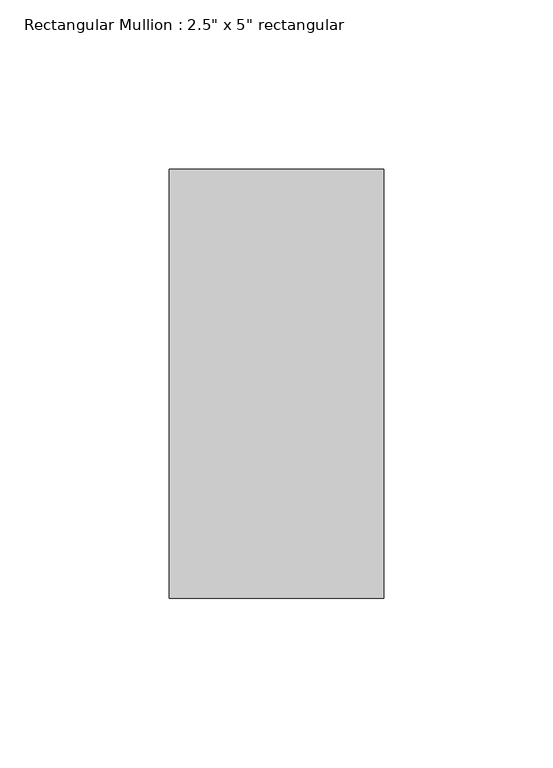
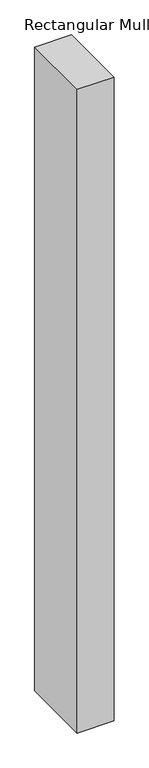
"""IFC4 building model written with IfcOpenShell, lengths in millimetres: member geometry."""

from ifc_helpers import new_model, si_unit, frame, origin, place, context, project, spatial, polyline, outline, extrude, source, transform, mapped, element, save


def member_f6bf76ec(model_context):
    return source(origin(), model_context, "Body", "SweptSolid", [
        extrude(outline(polyline([(0.0, 63.5), (0.0, -63.5), (-63.5, -63.5), (-63.5, 63.5), (0.0, 63.5)])), frame((0.0, 0.0, -1175.371271), z_axis=(0.0, 0.0, 1.0), x_axis=(1.0, 0.0, 0.0)), (0.0, 0.0, 1.0), 1175.371271),
    ])


if __name__ == "__main__":
    model = new_model("IFC4")
    model_context = context("Model", 3, world=origin())
    ifc_project = project(units=[si_unit("LENGTHUNIT", "METRE", prefix="MILLI")], contexts=[model_context])
    site = spatial("IfcSite", under=ifc_project)
    building = spatial("IfcBuilding", under=site)
    placement = place(None, origin())
    member_shape = member_f6bf76ec(model_context)
    element("IfcMember", 1, ObjectType="Rectangular Mullion : 2.5\" x 5\" rectangular", at=placement, inside=building, context=model_context, shape_type="MappedRepresentation", body=[
        mapped(member_shape, transform((0.0, 0.0, 0.0), x_axis=(1.0, 0.0, 0.0), y_axis=(0.0, 1.0, 0.0), z_axis=(0.0, 0.0, 1.0))),
    ])
    save(model, "model.ifc")

# Revit data of these elements
# Type "Rectangular Mullion : 2.5\" x 5\" rectangular"
#   built-in parameter 1007304 = 0.416667 (stored number, unit not read)
#   built-in parameter 1007301 = 0.104167 (stored number, unit not read)
#   built-in parameter 1007300 = 0.104167 (stored number, unit not read)
# Element 1 (IfcMember, "Rectangular Mullion : 2.5\" x 5\" rectangular")
#   Materials on its faces: "Aluminum"
# Materials
#   "Aluminum": class "Metal", colour RGB 247 247 247, transparency 0, Description = "Aluminum 6061", Cost = 0
